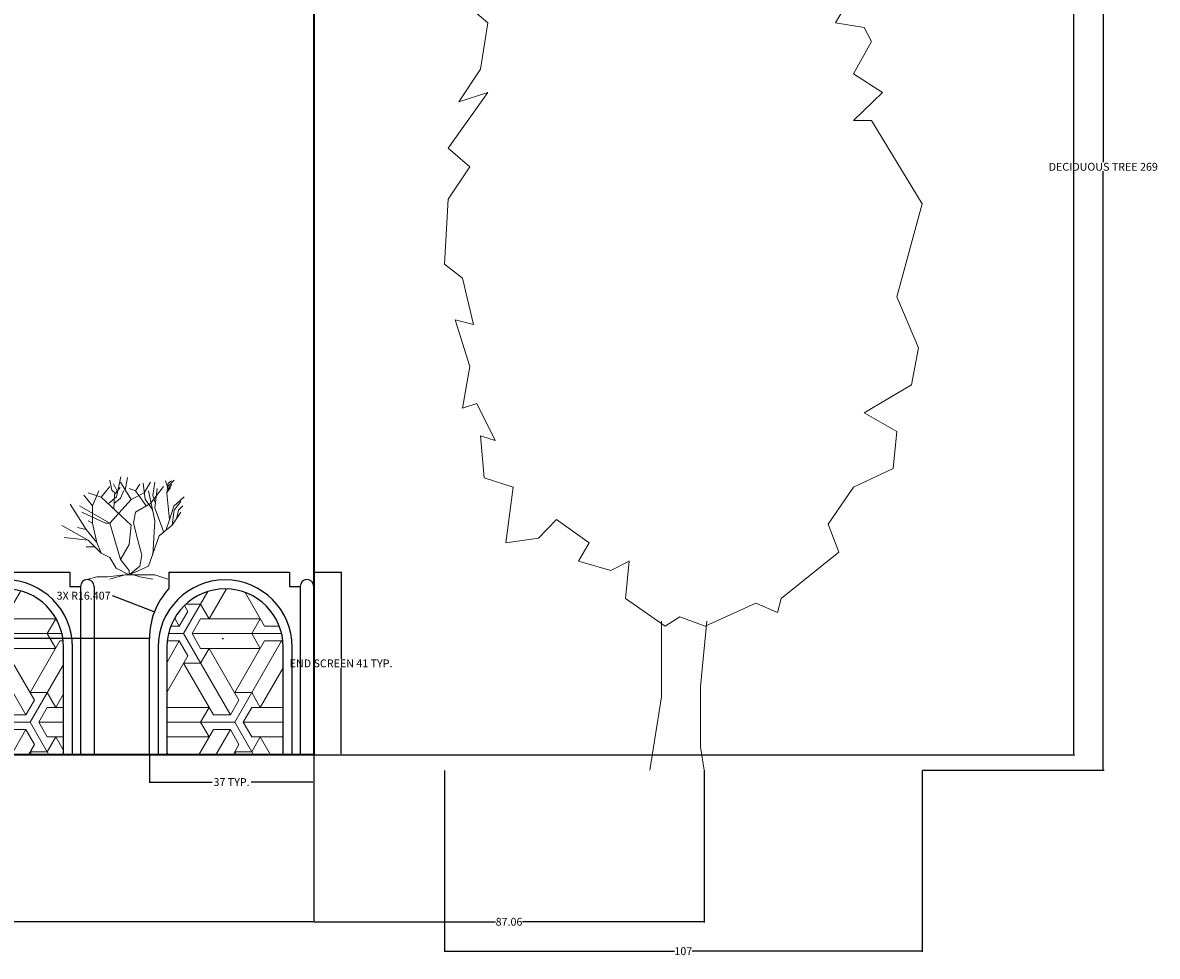
# Model space of a CAD drawing. Units: inches. Extents: x -17 to 741, y 7 to 490.
# Tile 7 of 8: x 489 to 741, y 7 to 215. Entities that reach past the tile are written whole.
import ezdxf

# ---------------------------------------------------------------- set-up
doc = ezdxf.new("R2010")
doc.units = ezdxf.units.IN
doc.header["$MEASUREMENT"] = 0
for name, color, linetype, lineweight in [('A-ANNO-DIMS', 2, 'Continuous', 18), ('A-WALL', 7, 'Continuous', 35), ('A-WALL-PATT', 8, 'Continuous', 13), ('A-WALL-SCRN', 7, 'Continuous', 25), ('L-PLNT', 3, 'Continuous', 18)]:
    doc.layers.add(name, color=color, linetype=linetype, lineweight=lineweight)
doc.styles.get("Standard").update_dxf_attribs({"font": 'arial.ttf'})
doc.dimstyles.get("Standard").update_dxf_attribs({"dimtxt": 1.75, "dimasz": 0.18, "dimexe": 0.18, "dimexo": 0.0625, "dimgap": 0.09, "dimtad": 0, "dimtih": 1, "dimtoh": 1, "dimdec": 4, "dimzin": 0, "dimdsep": 46, "dimlunit": 4, "dimtxsty": 'Standard', "dimcen": 0.09, "dimadec": 0, "dimazin": 0, "dimtfac": 1, "dimtdec": 4, "dimtofl": 0, "dimtmove": 0, "dimatfit": 3, "dimfxl": 1, "dimtolj": 1, "dimtzin": 0, "dimarcsym": 0})

# ---------------------------------------------------------------- blocks, each defined once
blk = doc.blocks.new('Shrub - elevation')
for p, q in [((-14.88, 18.24), (-12.96, 20.64)), ((-12.471, 19.775), (-12.898, 22.044)), ((-11.28, 19.619), (-12.104, 21.184)), ((-11.921, 18.836), (-10.64, 20.401)), ((-11.433, 18.289), (-10.457, 22.749)), ((-8.16, 17.76), (-10.56, 21.6)), ((-9.48, 19.775), (-8.992, 22.592)), ((-7.2, 19.68), (-6.24, 21.12)), ((-5.086, 17.741), (-5.513, 21.34)), ((-5.28, 19.2), (-3.84, 21.6)), ((-3.84, 16.8), (-0.96, 20.64)), ((-3.377, 18.602), (-2.888, 21.575)), ((-0.508, 21.888), (-0.081, 20.558)), ((-0.203, 19.149), (0.102, 21.34)), ((-0.142, 19.384), (0.59, 20.401)), ((-0.02, 20.01), (0.896, 21.105)), ((0.041, 20.714), (1.384, 22.044)), ((0.102, 21.34), (0.835, 21.888)), ((-16.8, 16.32), (-18.72, 18.72)), ((-14.88, 18.24), (-17.76, 19.2)), ((-16.8, 16.32), (-15.36, 19.68)), ((-8.16, 12), (-14.88, 18.24)), ((-13.325, 16.724), (-11.433, 18.289)), ((-12.96, 12.48), (-8.16, 17.76)), ((-11.677, 19.071), (-12.471, 19.775)), ((-12.043, 15.628), (-11.921, 18.836)), ((-11.982, 16.802), (-10.579, 18.054)), ((-10.579, 18.054), (-9.846, 19.697)), ((-7.2, 19.68), (-8.64, 20.16)), ((-8.16, 17.76), (-5.28, 19.2)), ((-4.8, 16.32), (-7.2, 19.68)), ((-3.377, 15.315), (-5.086, 17.819)), ((-2.88, 12.96), (-4.32, 19.68)), ((-2.766, 16.802), (-3.377, 18.602)), ((-2.88, 15.84), (-2.4, 20.16)), ((0.346, 13.203), (-0.203, 19.149)), ((1.323, 16.254), (3.642, 18.289)), ((-18.24, 11.04), (-21.755, 16.655)), ((-12.96, 12.48), (-19.68, 16.32)), ((-16.8, 12.48), (-16.8, 16.32)), ((-7.2, 14.88), (-3.84, 16.8)), ((-0.96, 10.56), (-2.88, 15.84)), ((0.346, 13.203), (1.323, 16.254)), ((0.96, 12), (1.44, 15.36)), ((1.44, 15.36), (2.88, 17.28)), ((1.92, 13.44), (2.4, 15.36)), ((2.4, 15.36), (3.36, 16.32)), ((-13.92, 12.48), (-19.2, 14.88)), ((-16.8, 12.48), (-17.76, 12.96)), ((-7.68, 12.48), (-7.2, 14.88)), ((-3.36, 5.28), (-2.88, 12.96)), ((-0.48, 10.8), (0.346, 13.203)), ((0.96, 12), (2.88, 14.88)), ((-17.76, 8.64), (-23.663, 11.961)), ((-18.24, 11.04), (-20.16, 11.52)), ((-15.84, 8.16), (-18.24, 11.04)), ((-15.84, 8.16), (-16.8, 12.48)), ((-12.96, 12.48), (-13.92, 12.48)), ((-10.56, 4.32), (-12.96, 12.48)), ((-8.64, 7.68), (-8.16, 12)), ((-6.72, 8.64), (-7.68, 12.48)), ((-1.92, 9.6), (0.96, 12)), ((-17.76, 8.64), (-23.128, 9.222)), ((-14.88, 5.76), (-17.76, 8.64)), ((-14.88, 5.76), (-15.84, 8.16)), ((-10.56, 4.32), (-8.64, 7.68)), ((-5.76, 5.28), (-6.72, 8.64)), ((-4.32, 2.88), (-1.92, 9.6)), ((-16.32, 7.2), (-18.24, 7.2)), ((-12.96, 4.8), (-14.88, 5.76)), ((-6.24, 2.88), (-5.76, 5.28)), ((-11.52, 2.4), (-12.96, 4.8)), ((-8.64, 1.92), (-10.56, 4.32)), ((-8.64, 0.96), (-4.32, 2.88)), ((-8.64, 0.96), (-6.24, 2.88)), ((-15.84, 0.48), (-17.76, 0)), ((-13.44, 0.48), (-15.84, 0.48)), ((-9.6, 0.96), (-13.44, 0.48)), ((-9.6, 0.96), (-12.96, 0)), ((-8.64, 0.96), (-11.52, 2.4)), ((-9.6, 0.96), (-7.68, 0.96)), ((-8.64, 0.96), (-8.64, 1.92)), ((-8.64, 0.96), (-2.88, 0.96)), ((-7.68, 0.96), (-6.24, 0.48)), ((-6.24, 0.48), (-3.36, 0)), ((-2.88, 0.96), (0, 0))]:
    blk.add_line(p, q)
blk = doc.blocks.new('Tree - type 2 deciduous elevation')
blk.add_lwpolyline([(-2.754, 191.699), (-6.78, 182.851), (-13.682, 176.953), (-11.956, 173.266), (-9.656, 172.529), (-14.257, 170.317), (-13.682, 167.368), (-21.733, 157.783), (-25.184, 154.834), (-21.158, 150.41), (-21.733, 147.461), (-22.884, 140.825), (-26.334, 140.087), (-29.21, 134.926), (-28.635, 129.028), (-32.661, 128.291), (-36.111, 120.18), (-34.386, 118.706), (-35.536, 111.333), (-38.987, 106.171), (-34.386, 107.646), (-40.712, 98.798), (-37.261, 95.849), (-40.712, 90.688), (-41.287, 80.366), (-38.412, 78.154), (-36.686, 70.781), (-39.562, 71.518), (-37.261, 64.145), (-38.412, 57.509), (-36.111, 58.247), (-33.236, 52.348), (-35.536, 53.086), (-34.961, 46.45), (-30.36, 44.975), (-31.51, 36.128), (-26.334, 36.865), (-23.459, 39.814), (-18.283, 36.128), (-20.008, 33.178), (-14.832, 31.704), (-11.956, 33.178), (-12.531, 27.28), (-6.205, 22.856), (-3.905, 24.331), (0.121, 22.856), (8.173, 26.543), (11.624, 25.068), (12.199, 27.28), (21.4, 34.653), (19.675, 39.077), (23.701, 44.975), (30.027, 47.924), (30.602, 53.823), (25.426, 56.772), (32.903, 61.196), (34.053, 67.094), (30.602, 75.205), (34.628, 89.951), (26.576, 103.222), (23.701, 103.222), (28.302, 107.646), (23.701, 110.595), (26.576, 115.756), (25.426, 117.968), (20.825, 118.706), (24.276, 124.604), (22.551, 137.876), (19.1, 139.35), (22.551, 140.825), (19.675, 151.884), (14.499, 153.359), (16.224, 162.207), (12.199, 170.317), (10.473, 167.368), (5.872, 179.165), (4.147, 177.69), (0.696, 187.275), (-0.454, 185.8)], close=True)
for points in [[(-6.813, 23.669), (-6.813, 11.669), (-8.627, 0)], [(0.387, 23.669), (-0.576, 13.271), (-0.576, 3.686), (0, 0)]]:
    blk.add_lwpolyline(points)
blk = doc.blocks.new('SCREEN-ARCH-END-BAY')
for p, q in [((4.33, 40.71), (4.33, 37.01)), ((4.33, 40.71), (31.23, 40.71)), ((31.23, 40.71), (31.23, 37.52)), ((31.23, 37.52), (33.14, 37.52)), ((33.14, 37.52), (33.61, 37.52)), ((33.61, 37.52), (33.61, 0)), ((36.63, 37.52), (36.63, 0)), ((0, 0), (0, 25.9))]:
    blk.add_line(p, q)
for points in [[(31.83, 0), (31.83, 24, 1), (1.92, 24), (1.92, 0)], [(29.83, 0), (29.83, 24, 1), (3.92, 24), (3.92, 0)]]:
    blk.add_lwpolyline(points, format="xyb")
for centre, radius, start in [((35.12, 37.52), 1.51, 0), ((16.41, 25.9), 16.41, 137.3839)]:
    blk.add_arc(centre, radius, start, 180)
blk = doc.blocks.new('*D19')
at = {"layer": 'A-ANNO-DIMS', "color": 0, "lineweight": -2, "transparency": 16777216}
for p, q in [((553.49, 92.72), (559.71, 92.72)), ((559.53, 92.54), (559.53, 73.36)), ((559.53, 52.19), (559.53, 71.37)), ((553.49, 52.01), (559.71, 52.01))]:
    blk.add_line(p, q, dxfattribs=at)
at = {"layer": 'A-ANNO-DIMS', "color": 0, "transparency": 16777216}
for points in [[(559.5, 92.54), (559.56, 92.54), (559.53, 92.72)], [(559.5, 52.19), (559.56, 52.19), (559.53, 52.01)]]:
    blk.add_solid(points, dxfattribs=at)
at = {"layer": 'Defpoints', "color": 0, "transparency": 16777216}
for p in [(553.43, 92.72), (559.53, 92.72), (553.43, 52.01)]:
    blk.add_point(p, dxfattribs=at)
at = {"layer": 'A-ANNO-DIMS', "color": 0, "transparency": 16777216, "insert": (559.53, 72.36), "char_height": 1.75, "attachment_point": 5}
blk.add_mtext('\\A1;END SCREEN 41 TYP.', dxfattribs=at)
blk = doc.blocks.new('*D20')
at = {"layer": 'A-ANNO-DIMS', "color": 0, "lineweight": -2, "transparency": 16777216}
for p, q in [((516.8, 51.95), (516.8, 45.72)), ((553.43, 51.95), (553.43, 45.72)), ((516.98, 45.9), (530.76, 45.9)), ((553.25, 45.9), (539.46, 45.9))]:
    blk.add_line(p, q, dxfattribs=at)
at = {"layer": 'A-ANNO-DIMS', "color": 0, "transparency": 16777216}
for points in [[(516.98, 45.93), (516.98, 45.87), (516.8, 45.9)], [(553.25, 45.93), (553.25, 45.87), (553.43, 45.9)]]:
    blk.add_solid(points, dxfattribs=at)
at = {"layer": 'Defpoints', "color": 0, "transparency": 16777216}
for p in [(516.8, 52.01), (553.43, 52.01), (553.43, 45.9)]:
    blk.add_point(p, dxfattribs=at)
at = {"layer": 'A-ANNO-DIMS', "color": 0, "transparency": 16777216, "insert": (535.11, 45.9), "char_height": 1.75, "attachment_point": 5}
blk.add_mtext('\\A1;37 TYP.', dxfattribs=at)
blk = doc.blocks.new('*D35')
at = {"layer": 'A-ANNO-DIMS', "color": 0, "lineweight": -2, "transparency": 16777216}
for p, q in [((689.15, 317.56), (729.61, 317.56)), ((729.43, 317.38), (729.43, 184.06)), ((729.43, 48.74), (729.43, 182.06)), ((689.15, 48.56), (729.61, 48.56))]:
    blk.add_line(p, q, dxfattribs=at)
at = {"layer": 'A-ANNO-DIMS', "color": 0, "transparency": 16777216}
for points in [[(729.4, 317.38), (729.46, 317.38), (729.43, 317.56)], [(729.4, 48.74), (729.46, 48.74), (729.43, 48.56)]]:
    blk.add_solid(points, dxfattribs=at)
at = {"layer": 'Defpoints', "color": 0, "transparency": 16777216}
for p in [(689.08, 317.56), (729.43, 317.56), (689.08, 48.56)]:
    blk.add_point(p, dxfattribs=at)
at = {"layer": 'A-ANNO-DIMS', "color": 0, "transparency": 16777216, "insert": (729.43, 183.06), "char_height": 1.75, "attachment_point": 5}
blk.add_mtext('\\A1;DECIDUOUS TREE 269', dxfattribs=at)
blk = doc.blocks.new('*D36')
at = {"layer": 'A-ANNO-DIMS', "color": 0, "lineweight": -2, "transparency": 16777216}
for p, q in [((582.56, 48.5), (582.56, 8.03)), ((689.08, 48.5), (689.08, 8.03)), ((582.74, 8.21), (633.88, 8.21)), ((688.9, 8.21), (637.76, 8.21))]:
    blk.add_line(p, q, dxfattribs=at)
at = {"layer": 'A-ANNO-DIMS', "color": 0, "transparency": 16777216}
for points in [[(582.74, 8.24), (582.74, 8.18), (582.56, 8.21)], [(688.9, 8.24), (688.9, 8.18), (689.08, 8.21)]]:
    blk.add_solid(points, dxfattribs=at)
at = {"layer": 'Defpoints', "color": 0, "transparency": 16777216}
for p in [(582.56, 48.56), (689.08, 48.56), (689.08, 8.21)]:
    blk.add_point(p, dxfattribs=at)
at = {"layer": 'A-ANNO-DIMS', "color": 0, "transparency": 16777216, "insert": (635.82, 8.21), "char_height": 1.75, "attachment_point": 5}
blk.add_mtext('\\A1;107', dxfattribs=at)
blk = doc.blocks.new('*D37')
at = {"layer": 'A-ANNO-DIMS', "color": 0, "lineweight": -2, "transparency": 16777216}
for p, q in [((20.52, 396.95), (20.52, 14.58)), ((553.43, 51.95), (553.43, 14.58)), ((20.7, 14.76), (283.93, 14.76)), ((553.25, 14.76), (290.02, 14.76))]:
    blk.add_line(p, q, dxfattribs=at)
at = {"layer": 'A-ANNO-DIMS', "color": 0, "transparency": 16777216}
for points in [[(20.7, 14.79), (20.7, 14.73), (20.52, 14.76)], [(553.25, 14.79), (553.25, 14.73), (553.43, 14.76)]]:
    blk.add_solid(points, dxfattribs=at)
at = {"layer": 'Defpoints', "color": 0, "transparency": 16777216}
for p in [(20.52, 397.01), (553.43, 52.01), (553.43, 14.76)]:
    blk.add_point(p, dxfattribs=at)
at = {"layer": 'A-ANNO-DIMS', "color": 0, "transparency": 16777216, "insert": (286.97, 14.76), "char_height": 1.75, "attachment_point": 5}
blk.add_mtext('\\A1;532.9', dxfattribs=at)
blk = doc.blocks.new('*D38')
at = {"layer": 'A-ANNO-DIMS', "color": 0, "lineweight": -2, "transparency": 16777216}
for p, q in [((341.83, 454.57), (723.06, 454.57)), ((722.88, 454.39), (722.88, 254.27)), ((722.88, 52.19), (722.88, 252.31)), ((553.49, 52.01), (723.06, 52.01))]:
    blk.add_line(p, q, dxfattribs=at)
at = {"layer": 'A-ANNO-DIMS', "color": 0, "transparency": 16777216}
for points in [[(722.85, 454.39), (722.91, 454.39), (722.88, 454.57)], [(722.85, 52.19), (722.91, 52.19), (722.88, 52.01)]]:
    blk.add_solid(points, dxfattribs=at)
at = {"layer": 'Defpoints', "color": 0, "transparency": 16777216}
for p in [(341.77, 454.57), (722.88, 454.57), (553.43, 52.01)]:
    blk.add_point(p, dxfattribs=at)
at = {"layer": 'A-ANNO-DIMS', "color": 0, "transparency": 16777216, "insert": (722.88, 253.29), "char_height": 1.75, "attachment_point": 5}
blk.add_mtext('\\A1;402.6', dxfattribs=at)
blk = doc.blocks.new('*D54')
at = {"layer": 'A-ANNO-DIMS', "color": 0, "lineweight": -2, "transparency": 16777216}
for p, q in [((458.05, 167.89), (458.05, 488.55)), ((458.23, 488.37), (502.69, 488.37)), ((553.25, 488.37), (508.78, 488.37)), ((553.43, 52.07), (553.43, 488.55))]:
    blk.add_line(p, q, dxfattribs=at)
at = {"layer": 'A-ANNO-DIMS', "color": 0, "transparency": 16777216}
for points in [[(458.23, 488.4), (458.23, 488.34), (458.05, 488.37)], [(553.25, 488.4), (553.25, 488.34), (553.43, 488.37)]]:
    blk.add_solid(points, dxfattribs=at)
at = {"layer": 'Defpoints', "color": 0, "transparency": 16777216}
for p in [(553.43, 488.37), (458.05, 167.83), (553.43, 52.01)]:
    blk.add_point(p, dxfattribs=at)
at = {"layer": 'A-ANNO-DIMS', "color": 0, "transparency": 16777216, "insert": (505.74, 488.37), "char_height": 1.75, "attachment_point": 5}
blk.add_mtext('\\A1;95.38', dxfattribs=at)
blk = doc.blocks.new('*D63')
at = {"layer": 'A-ANNO-DIMS', "color": 0, "lineweight": -2, "transparency": 16777216}
for p, q in [((553.43, 51.95), (553.43, 14.58)), ((640.49, 48.5), (640.49, 14.58)), ((553.61, 14.76), (593.92, 14.76)), ((640.31, 14.76), (600, 14.76))]:
    blk.add_line(p, q, dxfattribs=at)
at = {"layer": 'A-ANNO-DIMS', "color": 0, "transparency": 16777216}
for points in [[(553.61, 14.79), (553.61, 14.73), (553.43, 14.76)], [(640.31, 14.79), (640.31, 14.73), (640.49, 14.76)]]:
    blk.add_solid(points, dxfattribs=at)
at = {"layer": 'Defpoints', "color": 0, "transparency": 16777216}
for p in [(553.43, 52.01), (640.49, 48.56), (640.49, 14.76)]:
    blk.add_point(p, dxfattribs=at)
at = {"layer": 'A-ANNO-DIMS', "color": 0, "transparency": 16777216, "insert": (596.96, 14.76), "char_height": 1.75, "attachment_point": 5}
blk.add_mtext('\\A1;87.06', dxfattribs=at)
blk = doc.blocks.new('*D64')
at = {"layer": 'A-ANNO-DIMS', "color": 0, "lineweight": -2, "transparency": 16777216}
for p, q in [((516.74, 77.91), (-13.46, 77.91)), ((-13.28, 77.73), (-13.28, 65.94)), ((-13.28, 52.19), (-13.28, 63.98)), ((516.74, 52.01), (-13.46, 52.01))]:
    blk.add_line(p, q, dxfattribs=at)
at = {"layer": 'A-ANNO-DIMS', "color": 0, "transparency": 16777216}
for points in [[(-13.31, 77.73), (-13.25, 77.73), (-13.28, 77.91)], [(-13.31, 52.19), (-13.25, 52.19), (-13.28, 52.01)]]:
    blk.add_solid(points, dxfattribs=at)
at = {"layer": 'Defpoints', "color": 0, "transparency": 16777216}
for p in [(-13.28, 77.91), (516.8, 77.91), (516.8, 52.01)]:
    blk.add_point(p, dxfattribs=at)
at = {"layer": 'A-ANNO-DIMS', "color": 0, "transparency": 16777216, "insert": (-13.28, 64.96), "char_height": 1.75, "attachment_point": 5}
blk.add_mtext('\\A1;25.9', dxfattribs=at)
blk = doc.blocks.new('*D69')
at = {"layer": 'A-ANNO-DIMS', "color": 0, "lineweight": -2, "transparency": 16777216}
for p, q in [((508.57, 87.45), (508.75, 87.45)), ((508.75, 87.45), (517.75, 83.94)), ((533.11, 77.91), (533.29, 77.91)), ((533.2, 77.82), (533.2, 78))]:
    blk.add_line(p, q, dxfattribs=at)
at = {"layer": 'A-ANNO-DIMS', "color": 0, "transparency": 16777216}
blk.add_solid([(517.76, 83.96), (517.74, 83.91), (517.92, 83.87)], dxfattribs=at)
at = {"layer": 'Defpoints', "color": 0, "transparency": 16777216}
for p in [(517.92, 83.87), (533.2, 77.91)]:
    blk.add_point(p, dxfattribs=at)
at = {"layer": 'A-ANNO-DIMS', "color": 0, "transparency": 16777216, "insert": (502.13, 87.45), "char_height": 1.75, "attachment_point": 5}
blk.add_mtext('\\A1;3X R16.407', dxfattribs=at)

msp = doc.modelspace()

# ---------------------------------------------------------------- hatches: boundary and pattern name
at = {"layer": 'A-WALL-PATT'}
h = msp.add_hatch(dxfattribs=at)
h.set_pattern_fill('ESCHER', color=256, scale=19)
h.paths.add_polyline_path([(497.6481, 76.0082, 1), (471.7452, 76.0082), (471.7452, 52.0082), (497.6481, 52.0082)])
h.paths.add_polyline_path([(546.6242, 76.0082, 1), (520.7212, 76.0082), (520.7212, 52.0082), (546.6242, 52.0082)])

# ---------------------------------------------------------------- linework, layer by layer
at = {"layer": 'A-WALL'}
for p, q in [((553.4286, 379.9466), (553.4286, 52.0082)), ((553.4286, 52.0082), (466.6607, 52.0082))]:
    msp.add_line(p, q, dxfattribs=at)

# ---------------------------------------------------------------- block references
at = {"layer": 'A-WALL-SCRN'}
for p in [(467.8218, 52.008), (516.7979, 52.008)]:
    msp.add_blockref('SCREEN-ARCH-END-BAY', p, dxfattribs=at)
at = {"layer": 'L-PLNT', "xscale": 1.403243224327764, "yscale": 1.403243224327764, "zscale": 1.403243224327764}
msp.add_blockref('Tree - type 2 deciduous elevation', (640.4911, 48.5597), dxfattribs=at)
at = {"layer": 'L-PLNT'}
msp.add_blockref('Shrub - elevation', (520.904, 91.1684), dxfattribs=at)

# ---------------------------------------------------------------- dimensions: what is measured, and where the dimension line sits
at = {"layer": 'A-ANNO-DIMS'}
for base, p1, p2, override, picture, middle in [((553.4286, 488.3717), (458.0494, 167.8255), (553.4286, 52.0082), {"dimdec": 2, "dimlfac": 1, "dimrnd": 0, "dimzin": 0, "dimdsep": 46, "dimlunit": 2}, '*D54', (505.739, 488.3717)), ((553.4286, 14.7597), (20.5169, 397.0087), (553.4286, 52.0082), {"dimdec": 1, "dimlfac": 1, "dimrnd": 0, "dimzin": 0, "dimdsep": 46, "dimlunit": 2}, '*D37', (286.9727, 14.7597)), ((640.4911, 14.7597), (553.4286, 52.0082), (640.4911, 48.5597), {"dimdec": 2, "dimlfac": 1, "dimrnd": 0, "dimzin": 0, "dimdsep": 46, "dimlunit": 2}, '*D63', (596.9598, 14.7597)), ((689.0826, 8.2096), (582.5554, 48.5597), (689.0826, 48.5597), {"dimdec": 0, "dimlfac": 1, "dimrnd": 0, "dimzin": 0, "dimdsep": 46, "dimlunit": 2}, '*D36', (635.819, 8.2096))]:
    dim = msp.add_linear_dim(base=base, p1=p1, p2=p2, dimstyle='Standard', override=override, dxfattribs=at)
    dim.commit()
    dim.dimension.update_dxf_attribs({"geometry": picture, "text_midpoint": middle})
for base, p1, p2, picture, middle in [((722.8826, 454.5717), (553.4286, 52.0082), (341.7687, 454.5717), '*D38', (722.8826, 253.2899)), ((-13.2831, 77.9092), (516.7979, 52.0082), (516.7979, 77.9092), '*D64', (-13.2831, 64.9587))]:
    dim = msp.add_linear_dim(base=base, p1=p1, p2=p2, angle=90, dimstyle='Standard', override={"dimdec": 1, "dimlfac": 1, "dimrnd": 0, "dimzin": 0, "dimdsep": 46, "dimlunit": 2}, dxfattribs=at)
    dim.commit()
    dim.dimension.update_dxf_attribs({"geometry": picture, "text_midpoint": middle})
for base, p1, p2, text, picture, middle in [((729.4326, 317.56), (689.0826, 48.5597), (689.0826, 317.56), 'DECIDUOUS TREE <>', '*D35', (729.4326, 183.0598)), ((559.5349, 92.7171), (553.4286, 52.0082), (553.4286, 92.7171), 'END SCREEN <> TYP.', '*D19', (559.5349, 72.3627))]:
    dim = msp.add_linear_dim(base=base, p1=p1, p2=p2, angle=90, text=text, dimstyle='Standard', override={"dimdec": 0, "dimlfac": 1, "dimrnd": 0, "dimzin": 0, "dimdsep": 46, "dimlunit": 2}, dxfattribs=at)
    dim.commit()
    dim.dimension.update_dxf_attribs({"geometry": picture, "text_midpoint": middle})
dim = msp.add_radius_dim(center=(533.2048, 77.9092), mpoint=(517.9194, 83.8709), text='3X <>', dimstyle='Standard', override={"dimdec": 3, "dimlfac": 1, "dimrnd": 0, "dimzin": 0, "dimdsep": 46, "dimlunit": 2}, dxfattribs=at)
dim.commit()
dim.dimension.update_dxf_attribs({"geometry": '*D69', "text_midpoint": (502.1287, 87.4478), "dimtype": 164})
dim = msp.add_linear_dim(base=(553.4286, 45.9018), p1=(516.7979, 52.0082), p2=(553.4286, 52.0082), text='<> TYP.', dimstyle='Standard', override={"dimdec": 0, "dimlfac": 1, "dimrnd": 0, "dimzin": 0, "dimdsep": 46, "dimlunit": 2}, dxfattribs=at)
dim.commit()
dim.dimension.update_dxf_attribs({"geometry": '*D20', "text_midpoint": (535.1133, 45.9018)})

doc.saveas('drawing.dxf')
